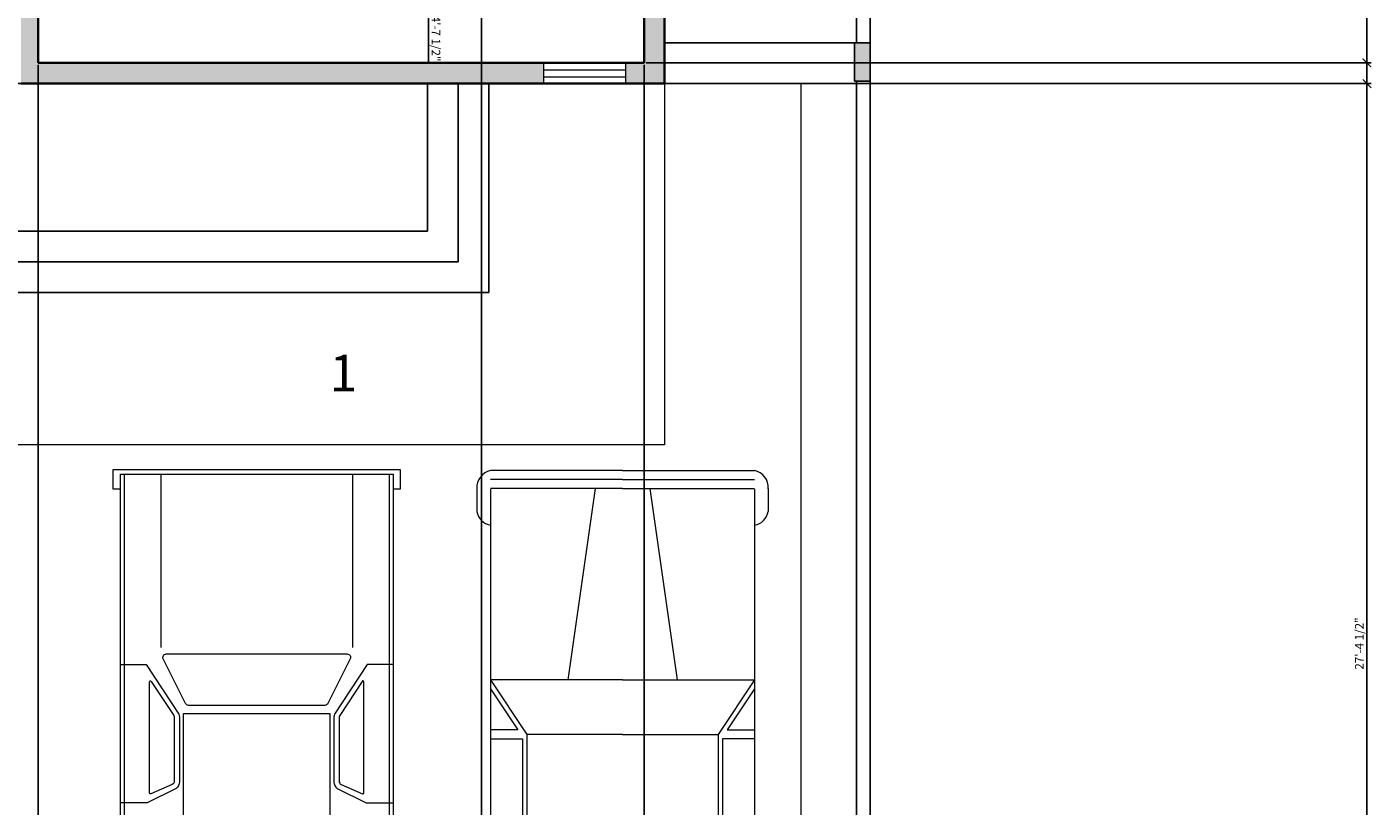
# Model space of a CAD drawing. Units: inches. Extents: x 3122 to 5933, y 1474 to 2995.
# Tile 10 of 12: x 5538 to 5933, y 2032 to 2261. Entities that reach past the tile are written whole.
import ezdxf

# ---------------------------------------------------------------- set-up
doc = ezdxf.new("R2010")
doc.units = ezdxf.units.IN
for name, color, linetype, lineweight in [('A-ANNO-DIMS', 2, 'Continuous', 18), ('A-AREA-IDEN', 7, 'Continuous', 20), ('A-DETL-PATT', 8, 'Continuous', 13), ('A-EQPM-VEHI', 8, 'Continuous', 13), ('A-FLOR-STRS', 7, 'Continuous', 25), ('A-GLAZ', 4, 'Continuous', 18), ('A-WALL', 7, 'Continuous', 35), ('A-WALL-PATT', 7, 'Continuous', 13), ('C-PROP', 7, 'Continuous', 25), ('C-SITE', 8, 'Continuous', 18)]:
    doc.layers.add(name, color=color, linetype=linetype, lineweight=lineweight)
doc.styles.get("Standard").update_dxf_attribs({"font": 'arial.ttf'})
doc.dimstyles.new('ISO-25', dxfattribs={"dimtxt": 2.5, "dimasz": 2.5, "dimexe": 1.25, "dimexo": 0.625, "dimtad": 1, "dimdec": 0, "dimlunit": 3, "dimtxsty": 'Standard', "dimblk": 'ARCHTICK', "dimcen": 2.5, "dimadec": 0, "dimazin": 0, "dimtfac": 1, "dimtdec": 0, "dimtmove": 0, "dimatfit": 3, "dimfxl": 1, "dimarcsym": 0})

# ---------------------------------------------------------------- blocks, each defined once
blk = doc.blocks.new('*U24')
for p, q in [((5.44, 42.31), (12.12, 42.31)), ((189.69, 42.31), (183.01, 42.31)), ((0.1, -0.41), (0.1, 38.35)), ((2.77, -0.41), (2.77, 38.31)), ((5.44, -0.41), (5.44, 38.24)), ((5.45, 38.31), (16.12, 38.31)), ((16.12, 38.31), (180.34, 38.31)), ((61.52, -0.41), (61.52, 38.31)), ((61.52, 38.31), (77.54, 27.62)), ((64.19, 38.31), (76.2, 30.29)), ((76.2, 30.29), (76.2, 38.31)), ((78.87, 38.31), (78.87, 28.96)), ((106.91, 28.96), (106.91, 38.31)), ((109.58, 27.62), (109.58, 38.31)), ((112.25, 38.31), (112.25, 28.96)), ((140.29, 28.96), (140.29, 38.31)), ((141.62, 27.62), (149.64, 38.31)), ((149.64, -0.41), (149.64, 38.31)), ((189.69, 38.31), (179.01, 38.31)), ((189.69, -0.41), (189.69, 38.24)), ((192.36, -0.41), (192.36, 38.31)), ((195.03, -0.41), (195.03, 38.35)), ((78.87, 28.96), (106.91, 28.96)), ((112.25, 28.96), (140.29, 28.96)), ((77.54, 27.62), (141.62, 27.62)), ((77.54, -0.41), (77.54, 27.62)), ((141.62, -0.41), (141.62, 27.62)), ((5.44, 7.6), (61.52, 15.61)), ((0.1, -0.42), (0.1, -39.18)), ((2.77, -0.41), (2.77, -39.13)), ((5.44, -0.42), (5.44, -39.07)), ((61.52, -0.41), (61.52, -39.13)), ((77.54, -0.41), (77.54, -28.45)), ((141.62, -0.41), (141.62, -28.45)), ((149.64, -0.41), (149.64, -39.13)), ((189.69, -0.42), (189.69, -39.07)), ((192.36, -0.41), (192.36, -39.13)), ((195.03, -0.42), (195.03, -39.18)), ((5.44, -8.42), (61.52, -16.43)), ((61.52, -39.13), (77.54, -28.45)), ((64.19, -39.13), (76.2, -31.12)), ((76.2, -31.12), (76.2, -39.13)), ((77.54, -28.45), (141.62, -28.45)), ((78.87, -39.13), (78.87, -29.79)), ((78.87, -29.79), (106.91, -29.79)), ((106.91, -29.79), (106.91, -39.13)), ((109.58, -28.45), (109.58, -39.13)), ((112.25, -29.79), (140.29, -29.79)), ((112.25, -39.13), (112.25, -29.79)), ((140.29, -29.79), (140.29, -39.13)), ((141.62, -28.45), (149.64, -39.13)), ((5.45, -39.13), (16.12, -39.13)), ((16.12, -39.13), (180.34, -39.13)), ((189.69, -39.13), (179.01, -39.13)), ((5.44, -43.14), (12.12, -43.14)), ((189.69, -43.14), (183.01, -43.14))]:
    blk.add_line(p, q)
for centre, radius, start, end in [((5.06, 37.26), 5.06, 85.6455, 168.0943), ((11.45, 37.64), 4.72, 8.1301, 81.87), ((183.68, 37.64), 4.72, 98.13, 171.8699), ((190.07, 37.26), 5.06, 11.9057, 94.3545), ((5.06, -38.09), 5.06, 191.9057, 274.3545), ((11.45, -38.46), 4.72, 278.13, 351.8699), ((183.68, -38.46), 4.72, 188.1301, 261.87), ((190.07, -38.09), 5.06, 265.6455, 348.0943)]:
    blk.add_arc(centre, radius, start, end)
blk = doc.blocks.new('*U36')
for p, q in [((1.28, 38.87), (175.66, 38.87)), ((1.28, 28.15), (52.13, 28.15)), ((1.28, -28.15), (52.13, -28.15)), ((1.28, -38.87), (175.66, -38.87))]:
    blk.add_line(p, q)
for points in [[(5.57, 40.01), (5.57, 42.18), (0, 42.18), (0, -42.18), (5.57, -42.18), (5.57, -40.01), (1.28, -40.01), (1.28, 40.01)], [(1.28, 40.01), (175.66, 40.01), (175.66, -40.01), (1.28, -40.01)], [(171.74, 40.01), (175.66, 40.01), (175.66, -40.01), (171.74, -40.01), (171.74, -42.18), (178.14, -42.18), (178.14, 42.18), (171.74, 42.18)], [(71.47, 21.48), (163.42, 21.48), (163.42, -21.48), (71.47, -21.48)]]:
    blk.add_lwpolyline(points, close=True)
for points in [[(57.15, 40.01), (57.15, 32.39), (71.72, 22.83, 0.086577), (72.56, 22.68), (91.59, 22.68, 0.227875), (93.54, 23.62), (97.72, 32.11), (97.72, 40.01)], [(57.15, -40.01), (57.15, -32.39), (71.72, -22.83, -0.086577), (72.56, -22.68), (91.59, -22.68, -0.227875), (93.54, -23.62), (97.72, -32.11), (97.72, -40.01)]]:
    blk.add_lwpolyline(points, format="xyb")
for points in [[(62.08, 30.95), (72.14, 24.35, 0.146139), (72.69, 24.18), (91.42, 24.18, 0.29766), (92.33, 24.78), (95.09, 31.05, 0.541236), (94.86, 31.41), (62.21, 31.41, 0.744989)], [(102.19, 24.58), (106.97, 31, -0.236929), (107.78, 31.41), (162.91, 31.41, -0.621576), (163.11, 31), (158.19, 24.58, -0.233368), (157.39, 24.18), (102.39, 24.18, -0.616908)], [(55.49, 27.42), (68.59, 20.89, -0.284287), (69.14, 19.99), (69.14, -19.99, -0.284287), (68.59, -20.89), (55.49, -27.42, -0.557284), (54.05, -26.53), (54.05, 26.53, -0.557284)], [(171.88, 27.31), (166.83, 24.47, 0.271143), (166.32, 23.6), (166.32, -23.6, 0.271143), (166.83, -24.47), (171.88, -27.31, 0.573387), (173.37, -26.44), (173.37, 26.44, 0.573387)], [(62.08, -30.95), (72.14, -24.35, -0.146139), (72.69, -24.18), (91.42, -24.18, -0.29766), (92.33, -24.78), (95.09, -31.05, -0.541236), (94.86, -31.41), (62.21, -31.41, -0.744989)], [(102.19, -24.58), (106.97, -31, 0.236929), (107.78, -31.41), (162.91, -31.41, 0.621576), (163.11, -31), (158.19, -24.58, 0.233368), (157.39, -24.18), (102.39, -24.18, 0.616908)]]:
    blk.add_lwpolyline(points, format="xyb", close=True)
blk = doc.blocks.new('_ArchTick')
at = {"color": 0, "linetype": 'ByBlock', "const_width": 0.15}
blk.add_lwpolyline([(-0.5, -0.5), (0.5, 0.5)], dxfattribs=at)
blk = doc.blocks.new('*D93')
at = {"layer": 'A-ANNO-DIMS', "color": 0, "lineweight": -2, "transparency": 16777216}
for p, q in [((5785.59, 2875.9), (5931.98, 2875.9)), ((5930.73, 1915.9), (5930.73, 2875.9)), ((5785.59, 1915.9), (5931.98, 1915.9))]:
    blk.add_line(p, q, dxfattribs=at)
at = {"layer": 'Defpoints', "color": 0, "transparency": 16777216}
for p in [(5784.96, 2875.9), (5930.73, 2875.9), (5784.96, 1915.9)]:
    blk.add_point(p, dxfattribs=at)
at = {"layer": 'A-ANNO-DIMS', "color": 0, "lineweight": -2, "transparency": 16777216, "xscale": 2.5, "yscale": 2.5, "zscale": 2.5}
for p, rotation in [((5930.73, 2875.9), 90), ((5930.73, 1915.9), 270)]:
    blk.add_blockref('_ArchTick', p, dxfattribs=dict(at, rotation=rotation))
at = {"layer": 'A-ANNO-DIMS', "color": 0, "transparency": 16777216, "insert": (5928.83, 2395.9), "char_height": 2.5, "attachment_point": 5, "rotation": 90}
blk.add_mtext('80\'-0"', dxfattribs=at)
blk = doc.blocks.new('*D106')
at = {"layer": 'A-ANNO-DIMS', "color": 0, "lineweight": -2, "transparency": 16777216}
for p, q in [((5540.87, 2249.87), (5540.87, 1792.93)), ((5718.65, 2249.87), (5718.65, 1792.93)), ((5540.87, 1794.18), (5718.65, 1794.18))]:
    blk.add_line(p, q, dxfattribs=at)
at = {"layer": 'Defpoints', "color": 0, "transparency": 16777216}
for p in [(5540.87, 2250.49), (5718.65, 2250.49), (5718.65, 1794.18)]:
    blk.add_point(p, dxfattribs=at)
at = {"layer": 'A-ANNO-DIMS', "color": 0, "lineweight": -2, "transparency": 16777216, "xscale": 2.5, "yscale": 2.5, "zscale": 2.5, "rotation": 180}
blk.add_blockref('_ArchTick', (5540.87, 1794.18), dxfattribs=at)
at = {"layer": 'A-ANNO-DIMS', "color": 0, "lineweight": -2, "transparency": 16777216, "xscale": 2.5, "yscale": 2.5, "zscale": 2.5}
blk.add_blockref('_ArchTick', (5718.65, 1794.18), dxfattribs=at)
at = {"layer": 'A-ANNO-DIMS', "color": 0, "transparency": 16777216, "insert": (5629.76, 1796.08), "char_height": 2.5, "attachment_point": 5}
blk.add_mtext('14\'-10"', dxfattribs=at)
blk = doc.blocks.new('*D107')
at = {"layer": 'A-ANNO-DIMS', "color": 0, "lineweight": -2, "transparency": 16777216}
for p, q in [((5719.28, 2532.69), (5931.98, 2532.69)), ((5930.73, 2250.49), (5930.73, 2532.69)), ((5719.28, 2250.49), (5931.98, 2250.49))]:
    blk.add_line(p, q, dxfattribs=at)
at = {"layer": 'Defpoints', "color": 0, "transparency": 16777216}
for p in [(5718.65, 2532.69), (5930.73, 2532.69), (5718.65, 2250.49)]:
    blk.add_point(p, dxfattribs=at)
at = {"layer": 'A-ANNO-DIMS', "color": 0, "lineweight": -2, "transparency": 16777216, "xscale": 2.5, "yscale": 2.5, "zscale": 2.5}
for p, rotation in [((5930.73, 2532.69), 90), ((5930.73, 2250.49), 270)]:
    blk.add_blockref('_ArchTick', p, dxfattribs=dict(at, rotation=rotation))
at = {"layer": 'A-ANNO-DIMS', "color": 0, "transparency": 16777216, "insert": (5928.83, 2391.59), "char_height": 2.5, "attachment_point": 5, "rotation": 90}
blk.add_mtext('23\'-6"', dxfattribs=at)
blk = doc.blocks.new('*D110')
at = {"layer": 'A-ANNO-DIMS', "color": 0, "lineweight": -2, "transparency": 16777216}
for p, q in [((5487.87, 2643.06), (5487.87, 1792.93)), ((5670.96, 2643.06), (5670.96, 1792.93)), ((5487.87, 1794.18), (5670.96, 1794.18))]:
    blk.add_line(p, q, dxfattribs=at)
at = {"layer": 'Defpoints', "color": 0, "transparency": 16777216}
for p in [(5487.87, 2643.69), (5670.96, 2643.69), (5670.96, 1794.18)]:
    blk.add_point(p, dxfattribs=at)
at = {"layer": 'A-ANNO-DIMS', "color": 0, "lineweight": -2, "transparency": 16777216, "xscale": 2.5, "yscale": 2.5, "zscale": 2.5, "rotation": 180}
blk.add_blockref('_ArchTick', (5487.87, 1794.18), dxfattribs=at)
at = {"layer": 'A-ANNO-DIMS', "color": 0, "lineweight": -2, "transparency": 16777216, "xscale": 2.5, "yscale": 2.5, "zscale": 2.5}
blk.add_blockref('_ArchTick', (5670.96, 1794.18), dxfattribs=at)
at = {"layer": 'A-ANNO-DIMS', "color": 0, "transparency": 16777216, "insert": (5579.42, 1796.09), "char_height": 2.5, "attachment_point": 5}
blk.add_mtext('15\'-3"', dxfattribs=at)
blk = doc.blocks.new('*D117')
at = {"layer": 'A-ANNO-DIMS', "color": 0, "lineweight": -2, "transparency": 16777216}
for p, q in [((5488.49, 2244.39), (5931.98, 2244.39)), ((5930.73, 1915.9), (5930.73, 2244.39)), ((5488.49, 1915.9), (5931.98, 1915.9))]:
    blk.add_line(p, q, dxfattribs=at)
at = {"layer": 'Defpoints', "color": 0, "transparency": 16777216}
for p in [(5487.87, 2244.39), (5930.73, 2244.39), (5487.87, 1915.9)]:
    blk.add_point(p, dxfattribs=at)
at = {"layer": 'A-ANNO-DIMS', "color": 0, "lineweight": -2, "transparency": 16777216, "xscale": 2.5, "yscale": 2.5, "zscale": 2.5}
for p, rotation in [((5930.73, 2244.39), 90), ((5930.73, 1915.9), 270)]:
    blk.add_blockref('_ArchTick', p, dxfattribs=dict(at, rotation=rotation))
at = {"layer": 'A-ANNO-DIMS', "color": 0, "transparency": 16777216, "insert": (5928.81, 2080.14), "char_height": 2.5, "attachment_point": 5, "rotation": 90}
blk.add_mtext('27\'-4 1/2"', dxfattribs=at)
blk = doc.blocks.new('*D130')
at = {"layer": 'A-ANNO-DIMS', "color": 0, "lineweight": -2, "transparency": 16777216}
for p in [(5655.34, 2349.62), (5655.34, 2250.26)]:
    blk.add_line(p, (5655.34, 2294.23), dxfattribs=at)
at = {"layer": 'Defpoints', "color": 0, "transparency": 16777216}
for p in [(5655.34, 2349.62), (5655.34, 2294.23)]:
    blk.add_point(p, dxfattribs=at)
at = {"layer": 'A-ANNO-DIMS', "color": 0, "lineweight": -2, "transparency": 16777216, "xscale": 2.5, "yscale": 2.5, "zscale": 2.5, "rotation": 90.0004117351408}
blk.add_blockref('_ArchTick', (5655.34, 2294.23), dxfattribs=at)
at = {"layer": 'A-ANNO-DIMS', "color": 0, "transparency": 16777216, "insert": (5657.26, 2261), "char_height": 2.5, "attachment_point": 5, "rotation": 270.0004}
blk.add_mtext('3X R4\'-7 1/2"', dxfattribs=at)

msp = doc.modelspace()

# ---------------------------------------------------------------- hatches: boundary and pattern name
at = {"layer": 'A-DETL-PATT'}
h = msp.add_hatch(color=256, dxfattribs=at)
h.dxf.hatch_style = 1
h.paths.add_polyline_path([(5784.96, 2256.39), (5780.41, 2256.39), (5780.41, 2245.15), (5784.96, 2245.15)])
at = {"layer": 'A-WALL-PATT'}
h = msp.add_hatch(color=256, dxfattribs=at)
h.dxf.hatch_style = 1
h.paths.add_polyline_path([(5536.42, 2643.69), (5487.87, 2643.69), (5487.87, 2667.06), (5485.81, 2667.06), (5481.87, 2667.06), (5481.87, 2643.69), (5481.87, 2590.35), (5487.87, 2590.35), (5487.87, 2634.69), (5524.65, 2634.69), (5524.65, 2538.69), (5487.87, 2538.69), (5487.87, 2554.35), (5481.87, 2554.35), (5481.87, 2532.69), (5524.65, 2532.69), (5658.65, 2532.69), (5718.65, 2532.69), (5718.65, 2501.93), (5724.65, 2501.93), (5724.65, 2549.4), (5718.65, 2549.4), (5718.65, 2538.69), (5658.65, 2538.69), (5658.65, 2573.57), (5658.59, 2573.63), (5654.65, 2573.63), (5654.65, 2538.69), (5594.65, 2538.69), (5594.65, 2573.57), (5594.59, 2573.63), (5590.65, 2573.63), (5590.65, 2538.69), (5530.65, 2538.69), (5530.65, 2634.69), (5536.42, 2634.69)])
h.paths.add_polyline_path([(5735.69, 2643.69), (5679.96, 2643.69), (5679.96, 2710.77), (5720.44, 2710.77), (5720.44, 2687.32), (5737.79, 2687.32), (5737.79, 2692.32), (5725.44, 2692.32), (5725.44, 2715.77), (5679.96, 2715.77), (5679.96, 2866.9), (5775.96, 2866.9), (5775.96, 2692.32), (5773.79, 2692.32), (5773.79, 2687.32), (5775.96, 2687.32), (5775.96, 2643.69), (5775.96, 2591.85), (5784.96, 2591.85), (5784.96, 2875.9), (5670.96, 2875.9), (5670.96, 2818.9), (5412.4, 2818.9), (5412.4, 2812.9), (5460.96, 2812.9), (5460.96, 2719.12), (5404.54, 2719.12), (5404.54, 2713.12), (5466.96, 2713.12), (5481.87, 2713.12), (5481.87, 2703.06), (5487.87, 2703.06), (5487.87, 2719.12), (5466.96, 2719.12), (5466.96, 2812.9), (5670.96, 2812.9), (5670.96, 2643.69), (5572.42, 2643.69), (5572.42, 2634.69), (5718.65, 2634.69), (5718.65, 2549.4), (5724.65, 2549.4), (5724.65, 2591.85), (5739.96, 2591.85), (5739.96, 2596.85), (5724.65, 2596.85), (5724.65, 2634.69), (5735.69, 2634.69)])
h.paths.add_polyline_path([(5594.65, 2634.69), (5590.65, 2634.69), (5590.65, 2603.63), (5594.65, 2603.63)], flags=17)
h.paths.add_polyline_path([(5724.65, 2441.93), (5718.65, 2441.93), (5718.65, 2336.51), (5724.65, 2336.51)])
h.paths.add_polyline_path([(5724.65, 2276.51), (5718.65, 2276.51), (5718.65, 2250.49), (5713.26, 2250.49), (5713.26, 2244.39), (5724.65, 2244.39)])
h.paths.add_polyline_path([(5689.26, 2250.49), (5540.87, 2250.49), (5540.87, 2317.46), (5535.87, 2317.46), (5535.87, 2244.39), (5689.26, 2244.39)])
h.paths.add_polyline_path([(5540.87, 2532.69), (5535.87, 2532.69), (5535.87, 2472.78), (5540.87, 2472.78)])
h.paths.add_polyline_path([(5540.87, 2472.78), (5537.87, 2472.78), (5537.87, 2346.69), (5537.87, 2317.46), (5540.87, 2317.46)])

# ---------------------------------------------------------------- linework, layer by layer
at = {"layer": 'A-FLOR-STRS'}
for p, q in [((5724.65, 2256.39), (5780.96, 2256.39)), ((5655.13, 2244.39), (5655.13, 2201.13)), ((5664.13, 2244.39), (5664.13, 2192.13)), ((5673.13, 2244.39), (5673.13, 2183.13)), ((5724.65, 2244.39), (5780.96, 2244.39)), ((5655.13, 2201.13), (5487.87, 2201.13)), ((5664.13, 2192.13), (5487.87, 2192.13)), ((5673.13, 2183.13), (5487.87, 2183.13))]:
    msp.add_line(p, q, dxfattribs=at)
at = {"layer": 'A-GLAZ'}
for p, q in [((5689.26, 2244.39), (5689.26, 2250.49)), ((5689.26, 2248.49), (5713.26, 2248.49)), ((5713.26, 2244.39), (5713.26, 2250.49)), ((5689.26, 2246.39), (5713.26, 2246.39))]:
    msp.add_line(p, q, dxfattribs=at)
at = {"layer": 'A-WALL'}
for p, q in [((5724.65, 2591.85), (5724.65, 2244.39)), ((5540.87, 2532.69), (5540.87, 2250.49)), ((5718.65, 2532.69), (5718.65, 2250.49)), ((5540.87, 2250.49), (5718.65, 2250.49)), ((5535.87, 2244.39), (5724.65, 2244.39))]:
    msp.add_line(p, q, dxfattribs=at)
at = {"layer": 'C-PROP'}
for p, q in [((5784.96, 1915.9), (5784.96, 2875.9)), ((5780.96, 2256.39), (5780.96, 2591.85)), ((5780.96, 1915.9), (5780.96, 2245.15))]:
    msp.add_line(p, q, dxfattribs=at)
msp.add_lwpolyline([(5780.41, 2256.39), (5784.96, 2256.39), (5784.96, 2245.15), (5780.41, 2245.15)], close=True, dxfattribs=at)
at = {"layer": 'C-SITE'}
for p, q in [((5724.65, 2244.39), (5724.65, 2138.47)), ((5764.72, 1915.9), (5764.72, 2244.39)), ((5724.65, 2138.47), (5487.87, 2138.47))]:
    msp.add_line(p, q, dxfattribs=at)

# ---------------------------------------------------------------- block references
at = {"layer": 'A-EQPM-VEHI', "rotation": 270}
for name, p in [('*U36', (5604.98, 2131.12)), ('*U24', (5712.74, 2131.01))]:
    msp.add_blockref(name, p, dxfattribs=at)

# ---------------------------------------------------------------- texts
at = {"layer": 'A-AREA-IDEN'}
msp.add_text('1', height=10.72, rotation=0.0333, dxfattribs=at).set_placement((5626.36, 2154.11))

# ---------------------------------------------------------------- dimensions: what is measured, and where the dimension line sits
at = {"layer": 'A-ANNO-DIMS'}
for base, p1, p2, picture, middle in [((5930.73, 2875.9), (5784.96, 1915.9), (5784.96, 2875.9), '*D93', (5928.83, 2395.9)), ((5930.73, 2532.69), (5718.65, 2250.49), (5718.65, 2532.69), '*D107', (5928.83, 2391.59)), ((5930.73, 2244.39), (5487.87, 1915.9), (5487.87, 2244.39), '*D117', (5928.81, 2080.14))]:
    dim = msp.add_linear_dim(base=base, p1=p1, p2=p2, angle=90, dimstyle='ISO-25', override={"dimdec": 1, "dimlfac": 1, "dimrnd": 0, "dimzin": 1, "dimdsep": 46, "dimlunit": 4, "dimfrac": 2}, dxfattribs=at)
    dim.commit()
    dim.dimension.update_dxf_attribs({"geometry": picture, "text_midpoint": middle})
for base, p1, p2, picture, middle in [((5670.96, 1794.18), (5487.87, 2643.69), (5670.96, 2643.69), '*D110', (5579.42, 1796.09)), ((5718.65, 1794.18), (5540.87, 2250.49), (5718.65, 2250.49), '*D106', (5629.76, 1796.08))]:
    dim = msp.add_linear_dim(base=base, p1=p1, p2=p2, dimstyle='ISO-25', override={"dimdec": 1, "dimlfac": 1, "dimrnd": 0, "dimzin": 1, "dimdsep": 46, "dimlunit": 4, "dimfrac": 2}, dxfattribs=at)
    dim.commit()
    dim.dimension.update_dxf_attribs({"geometry": picture, "text_midpoint": middle})
dim = msp.add_radius_dim(center=(5655.34, 2349.62), mpoint=(5655.34, 2294.23), text='3X <>', dimstyle='ISO-25', override={"dimdec": 1, "dimlfac": 1, "dimrnd": 0, "dimzin": 1, "dimdsep": 46, "dimlunit": 4, "dimfrac": 2}, dxfattribs=at)
dim.commit()
dim.dimension.update_dxf_attribs({"geometry": '*D130', "text_midpoint": (5655.34, 2261), "dimtype": 164})

doc.saveas('drawing.dxf')
